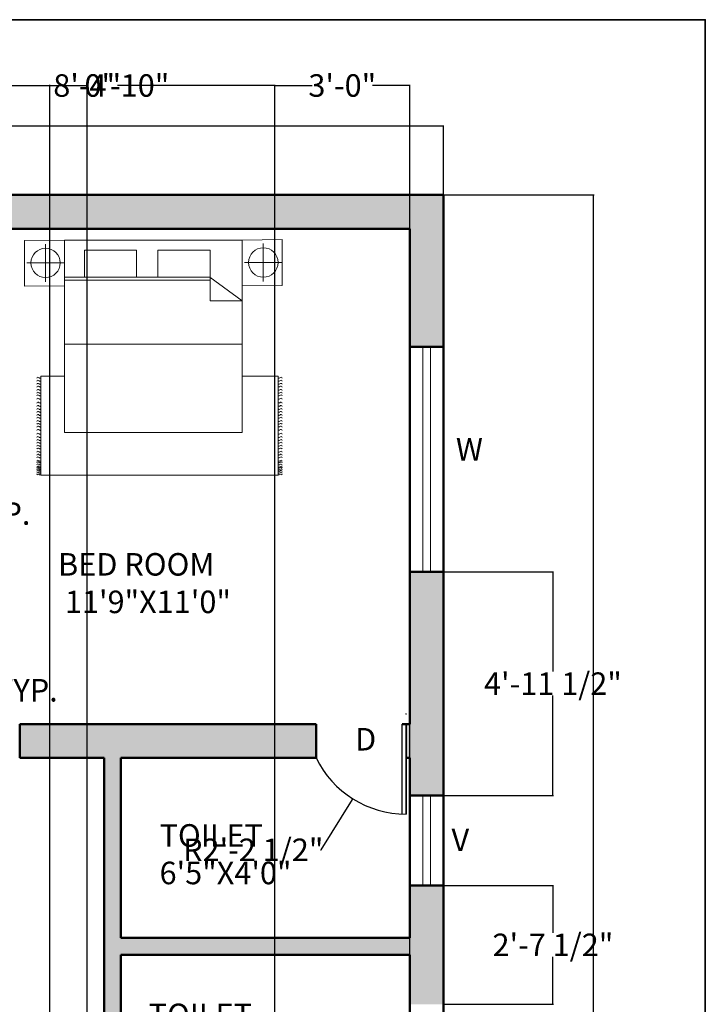
# Model space of a CAD drawing. Units: inches. Extents: x 125920 to 126336, y 366134 to 366735.
# Tile 6 of 6: x 126153 to 126336, y 366473 to 366735. Entities that reach past the tile are written whole.
import ezdxf

# ---------------------------------------------------------------- set-up
doc = ezdxf.new("R2010")
doc.units = ezdxf.units.IN
doc.header["$MEASUREMENT"] = 0
for name, color, linetype, lineweight in [('A-ANNO-DIMS', 2, 'Continuous', 18), ('A-ANNO-TEXT', 7, 'Continuous', 18), ('A-ANNO-TTLB', 7, 'Continuous', 35), ('A-AREA-IDEN', 7, 'Continuous', 25), ('A-DOOR', 3, 'Continuous', 25), ('A-FURN', 8, 'Continuous', 18), ('A-GLAZ', 4, 'Continuous', 18), ('A-WALL', 7, 'Continuous', 50)]:
    doc.layers.add(name, color=color, linetype=linetype, lineweight=lineweight)
doc.layers.add('A-WALL-PATT', color=18, linetype='Continuous', lineweight=13, true_color=0x000000)
doc.styles.get("Standard").update_dxf_attribs({"font": 'arial.ttf'})
doc.dimstyles.get("Standard").update_dxf_attribs({"dimtxt": 6, "dimasz": 0.18, "dimexe": 0.18, "dimexo": 0.0625, "dimgap": 0.09, "dimtad": 0, "dimtih": 1, "dimtoh": 1, "dimdec": 1, "dimzin": 0, "dimdsep": 46, "dimlunit": 3, "dimtxsty": 'Standard', "dimcen": 0.09, "dimadec": 0, "dimazin": 0, "dimtfac": 1, "dimtdec": 1, "dimtofl": 0, "dimtmove": 0, "dimatfit": 3, "dimfxl": 1, "dimtolj": 1, "dimtzin": 0, "dimarcsym": 0})

# ---------------------------------------------------------------- blocks, each defined once
blk = doc.blocks.new('*D3')
at = {"layer": 'A-ANNO-DIMS', "color": 0, "lineweight": -2, "transparency": 16777216}
for p, q in [((125966.47, 366688.86), (125966.47, 366707.25)), ((125966.65, 366707.07), (126111.24, 366707.07)), ((126266.29, 366707.07), (126121.71, 366707.07)), ((126266.47, 366688.86), (126266.47, 366707.25))]:
    blk.add_line(p, q, dxfattribs=at)
at = {"layer": 'A-ANNO-DIMS', "color": 0, "transparency": 16777216}
for points in [[(125966.65, 366707.1), (125966.65, 366707.04), (125966.47, 366707.07)], [(126266.29, 366707.1), (126266.29, 366707.04), (126266.47, 366707.07)]]:
    blk.add_solid(points, dxfattribs=at)
at = {"layer": 'Defpoints', "color": 0, "transparency": 16777216}
for p in [(126266.47, 366707.07), (125966.47, 366688.79), (126266.47, 366688.79)]:
    blk.add_point(p, dxfattribs=at)
at = {"layer": 'A-ANNO-DIMS', "color": 0, "transparency": 16777216, "insert": (126116.47, 366707.07), "char_height": 6, "attachment_point": 5}
blk.add_mtext("\\A1;25'", dxfattribs=at)
blk = doc.blocks.new('*D4')
at = {"layer": 'A-ANNO-DIMS', "color": 0, "lineweight": -2, "transparency": 16777216}
for p, q in [((126266.54, 366688.79), (126306.57, 366688.79)), ((126306.39, 366688.61), (126306.39, 366451.45)), ((126306.39, 366207.97), (126306.39, 366445.14)), ((126266.54, 366207.79), (126306.57, 366207.79))]:
    blk.add_line(p, q, dxfattribs=at)
at = {"layer": 'A-ANNO-DIMS', "color": 0, "transparency": 16777216}
for points in [[(126306.36, 366688.61), (126306.42, 366688.61), (126306.39, 366688.79)], [(126306.36, 366207.97), (126306.42, 366207.97), (126306.39, 366207.79)]]:
    blk.add_solid(points, dxfattribs=at)
at = {"layer": 'Defpoints', "color": 0, "transparency": 16777216}
for p in [(126266.47, 366688.79), (126266.47, 366207.79), (126306.39, 366207.79)]:
    blk.add_point(p, dxfattribs=at)
at = {"layer": 'A-ANNO-DIMS', "color": 0, "transparency": 16777216, "insert": (126306.39, 366448.29), "char_height": 6, "attachment_point": 5}
blk.add_mtext('\\A1;40\'-1.0"', dxfattribs=at)
blk = doc.blocks.new('BED-DOUBLE-WITH-NIGHTSTANDS')
for p, q in [((5.6, 61.62), (5.6, 51.56)), ((63.65, 61.72), (63.65, 51.66)), ((10.63, 56.59), (0.57, 56.59)), ((68.68, 56.69), (58.62, 56.69)), ((49.39, 52.82), (10.63, 52.82)), ((49.39, 52.82), (58, 46.47)), ((49.44, 52.82), (49.44, 46.47)), ((49.44, 52), (10.63, 52)), ((49.44, 46.47), (58, 46.47)), ((58.05, 34.96), (10.63, 34.96)), ((4.36, 0), (4.36, 26.37)), ((4.36, 26.37), (10.65, 26.37)), ((58.05, 26.37), (67.59, 26.37)), ((67.59, 26.37), (67.59, 0)), ((67.59, 0), (4.36, 0))]:
    blk.add_line(p, q)
for points in [[(0, 50.39), (10.63, 50.5), (10.63, 62.68), (0, 62.58)], [(58.05, 62.68), (58.05, 11.37), (10.63, 11.37), (10.63, 62.68)], [(58.05, 50.5), (68.68, 50.6), (68.68, 62.78), (58.05, 62.68)], [(29.88, 59.98), (29.88, 52.82), (15.98, 52.82), (15.98, 59.98)], [(49.44, 59.98), (49.44, 52.82), (35.55, 52.82), (35.55, 59.98)]]:
    blk.add_lwpolyline(points, close=True)
for centre in [(5.6, 56.59), (63.65, 56.69)]:
    blk.add_circle(centre, 3.92)
for points, knots in [([(3.23, 25.84), (3.32, 25.96), (3.52, 26.2), (3.86, 25.96), (4.14, 25.78), (4.29, 25.89), (4.36, 25.94)], [0, 0, 0, 0, 0.400747, 0.791423, 1.067667, 1.29709, 1.29709, 1.29709, 1.29709]), ([(3.23, 25.06), (3.32, 25.18), (3.52, 25.42), (3.86, 25.18), (4.14, 25.01), (4.29, 25.11), (4.36, 25.16)], [0, 0, 0, 0, 0.400747, 0.791423, 1.067667, 1.29709, 1.29709, 1.29709, 1.29709]), ([(3.23, 24.24), (3.32, 24.36), (3.52, 24.6), (3.86, 24.36), (4.14, 24.19), (4.29, 24.3), (4.36, 24.34)], [0, 0, 0, 0, 0.400747, 0.791423, 1.067667, 1.29709, 1.29709, 1.29709, 1.29709]), ([(3.23, 23.51), (3.32, 23.63), (3.52, 23.87), (3.86, 23.63), (4.14, 23.46), (4.29, 23.57), (4.36, 23.62)], [0, 0, 0, 0, 0.400747, 0.791423, 1.067667, 1.29709, 1.29709, 1.29709, 1.29709]), ([(68.71, 25.84), (68.61, 25.96), (68.42, 26.2), (68.08, 25.96), (67.8, 25.78), (67.65, 25.89), (67.58, 25.94)], [0, 0, 0, 0, 0.400747, 0.791423, 1.067667, 1.29709, 1.29709, 1.29709, 1.29709]), ([(68.71, 25.06), (68.61, 25.18), (68.42, 25.42), (68.08, 25.18), (67.8, 25.01), (67.65, 25.11), (67.58, 25.16)], [0, 0, 0, 0, 0.400747, 0.791423, 1.067667, 1.29709, 1.29709, 1.29709, 1.29709]), ([(68.71, 24.24), (68.61, 24.36), (68.42, 24.6), (68.08, 24.36), (67.8, 24.19), (67.65, 24.3), (67.58, 24.34)], [0, 0, 0, 0, 0.400747, 0.791423, 1.067667, 1.29709, 1.29709, 1.29709, 1.29709]), ([(68.71, 23.51), (68.61, 23.63), (68.42, 23.87), (68.08, 23.63), (67.8, 23.46), (67.65, 23.57), (67.58, 23.62)], [0, 0, 0, 0, 0.400747, 0.791423, 1.067667, 1.29709, 1.29709, 1.29709, 1.29709]), ([(3.23, 22.63), (3.32, 22.75), (3.52, 22.99), (3.86, 22.75), (4.14, 22.58), (4.29, 22.69), (4.36, 22.73)], [0, 0, 0, 0, 0.400747, 0.791423, 1.067667, 1.29709, 1.29709, 1.29709, 1.29709]), ([(3.23, 21.88), (3.32, 22), (3.52, 22.24), (3.86, 22), (4.14, 21.83), (4.29, 21.93), (4.36, 21.98)], [0, 0, 0, 0, 0.400747, 0.791423, 1.067667, 1.29709, 1.29709, 1.29709, 1.29709]), ([(3.23, 21.15), (3.32, 21.27), (3.52, 21.51), (3.86, 21.27), (4.14, 21.1), (4.29, 21.21), (4.36, 21.25)], [0, 0, 0, 0, 0.400747, 0.791423, 1.067667, 1.29709, 1.29709, 1.29709, 1.29709]), ([(68.71, 22.63), (68.61, 22.75), (68.42, 22.99), (68.08, 22.75), (67.8, 22.58), (67.65, 22.69), (67.58, 22.73)], [0, 0, 0, 0, 0.400747, 0.791423, 1.067667, 1.29709, 1.29709, 1.29709, 1.29709]), ([(68.71, 21.88), (68.61, 22), (68.42, 22.24), (68.08, 22), (67.8, 21.83), (67.65, 21.93), (67.58, 21.98)], [0, 0, 0, 0, 0.400747, 0.791423, 1.067667, 1.29709, 1.29709, 1.29709, 1.29709]), ([(68.71, 21.15), (68.61, 21.27), (68.42, 21.51), (68.08, 21.27), (67.8, 21.1), (67.65, 21.21), (67.58, 21.25)], [0, 0, 0, 0, 0.400747, 0.791423, 1.067667, 1.29709, 1.29709, 1.29709, 1.29709]), ([(3.23, 20.27), (3.32, 20.39), (3.52, 20.63), (3.86, 20.39), (4.14, 20.22), (4.29, 20.32), (4.36, 20.37)], [0, 0, 0, 0, 0.400747, 0.791423, 1.067667, 1.29709, 1.29709, 1.29709, 1.29709]), ([(3.23, 19.23), (3.32, 19.35), (3.52, 19.59), (3.86, 19.35), (4.14, 19.18), (4.29, 19.29), (4.36, 19.33)], [0, 0, 0, 0, 0.400747, 0.791423, 1.067667, 1.29709, 1.29709, 1.29709, 1.29709]), ([(3.23, 18.35), (3.32, 18.47), (3.52, 18.71), (3.86, 18.47), (4.14, 18.3), (4.29, 18.4), (4.36, 18.45)], [0, 0, 0, 0, 0.400747, 0.791423, 1.067667, 1.29709, 1.29709, 1.29709, 1.29709]), ([(68.71, 20.27), (68.61, 20.39), (68.42, 20.63), (68.08, 20.39), (67.8, 20.22), (67.65, 20.32), (67.58, 20.37)], [0, 0, 0, 0, 0.400747, 0.791423, 1.067667, 1.29709, 1.29709, 1.29709, 1.29709]), ([(68.71, 19.23), (68.61, 19.35), (68.42, 19.59), (68.08, 19.35), (67.8, 19.18), (67.65, 19.29), (67.58, 19.33)], [0, 0, 0, 0, 0.400747, 0.791423, 1.067667, 1.29709, 1.29709, 1.29709, 1.29709]), ([(68.71, 18.35), (68.61, 18.47), (68.42, 18.71), (68.08, 18.47), (67.8, 18.3), (67.65, 18.4), (67.58, 18.45)], [0, 0, 0, 0, 0.400747, 0.791423, 1.067667, 1.29709, 1.29709, 1.29709, 1.29709]), ([(3.23, 17.53), (3.32, 17.65), (3.52, 17.89), (3.86, 17.65), (4.14, 17.48), (4.29, 17.59), (4.36, 17.64)], [0, 0, 0, 0, 0.400747, 0.791423, 1.067667, 1.29709, 1.29709, 1.29709, 1.29709]), ([(3.23, 16.76), (3.32, 16.88), (3.52, 17.12), (3.86, 16.88), (4.14, 16.7), (4.29, 16.81), (4.36, 16.86)], [0, 0, 0, 0, 0.400747, 0.791423, 1.067667, 1.29709, 1.29709, 1.29709, 1.29709]), ([(3.23, 15.94), (3.32, 16.06), (3.52, 16.3), (3.86, 16.06), (4.14, 15.89), (4.29, 16), (4.36, 16.04)], [0, 0, 0, 0, 0.400747, 0.791423, 1.067667, 1.29709, 1.29709, 1.29709, 1.29709]), ([(68.71, 17.53), (68.61, 17.65), (68.42, 17.89), (68.08, 17.65), (67.8, 17.48), (67.65, 17.59), (67.58, 17.64)], [0, 0, 0, 0, 0.400747, 0.791423, 1.067667, 1.29709, 1.29709, 1.29709, 1.29709]), ([(68.71, 16.76), (68.61, 16.88), (68.42, 17.12), (68.08, 16.88), (67.8, 16.7), (67.65, 16.81), (67.58, 16.86)], [0, 0, 0, 0, 0.400747, 0.791423, 1.067667, 1.29709, 1.29709, 1.29709, 1.29709]), ([(68.71, 15.94), (68.61, 16.06), (68.42, 16.3), (68.08, 16.06), (67.8, 15.89), (67.65, 16), (67.58, 16.04)], [0, 0, 0, 0, 0.400747, 0.791423, 1.067667, 1.29709, 1.29709, 1.29709, 1.29709]), ([(3.23, 15.21), (3.32, 15.33), (3.52, 15.57), (3.86, 15.33), (4.14, 15.16), (4.29, 15.27), (4.36, 15.32)], [0, 0, 0, 0, 0.400747, 0.791423, 1.067667, 1.29709, 1.29709, 1.29709, 1.29709]), ([(3.23, 14.33), (3.32, 14.45), (3.52, 14.69), (3.86, 14.45), (4.14, 14.28), (4.29, 14.38), (4.36, 14.43)], [0, 0, 0, 0, 0.400747, 0.791423, 1.067667, 1.29709, 1.29709, 1.29709, 1.29709]), ([(3.23, 13.58), (3.32, 13.7), (3.52, 13.94), (3.86, 13.7), (4.14, 13.53), (4.29, 13.63), (4.36, 13.68)], [0, 0, 0, 0, 0.400747, 0.791423, 1.067667, 1.29709, 1.29709, 1.29709, 1.29709]), ([(3.23, 12.85), (3.32, 12.97), (3.52, 13.21), (3.86, 12.97), (4.14, 12.8), (4.29, 12.9), (4.36, 12.95)], [0, 0, 0, 0, 0.400747, 0.791423, 1.067667, 1.29709, 1.29709, 1.29709, 1.29709]), ([(68.71, 15.21), (68.61, 15.33), (68.42, 15.57), (68.08, 15.33), (67.8, 15.16), (67.65, 15.27), (67.58, 15.32)], [0, 0, 0, 0, 0.400747, 0.791423, 1.067667, 1.29709, 1.29709, 1.29709, 1.29709]), ([(68.71, 14.33), (68.61, 14.45), (68.42, 14.69), (68.08, 14.45), (67.8, 14.28), (67.65, 14.38), (67.58, 14.43)], [0, 0, 0, 0, 0.400747, 0.791423, 1.067667, 1.29709, 1.29709, 1.29709, 1.29709]), ([(68.71, 13.58), (68.61, 13.7), (68.42, 13.94), (68.08, 13.7), (67.8, 13.53), (67.65, 13.63), (67.58, 13.68)], [0, 0, 0, 0, 0.400747, 0.791423, 1.067667, 1.29709, 1.29709, 1.29709, 1.29709]), ([(68.71, 12.85), (68.61, 12.97), (68.42, 13.21), (68.08, 12.97), (67.8, 12.8), (67.65, 12.9), (67.58, 12.95)], [0, 0, 0, 0, 0.400747, 0.791423, 1.067667, 1.29709, 1.29709, 1.29709, 1.29709]), ([(3.23, 11.97), (3.32, 12.09), (3.52, 12.33), (3.86, 12.09), (4.14, 11.92), (4.29, 12.02), (4.36, 12.07)], [0, 0, 0, 0, 0.400747, 0.791423, 1.067667, 1.29709, 1.29709, 1.29709, 1.29709]), ([(3.23, 10.93), (3.32, 11.05), (3.52, 11.29), (3.86, 11.05), (4.14, 10.88), (4.29, 10.99), (4.36, 11.03)], [0, 0, 0, 0, 0.400747, 0.791423, 1.067667, 1.29709, 1.29709, 1.29709, 1.29709]), ([(68.71, 11.97), (68.61, 12.09), (68.42, 12.33), (68.08, 12.09), (67.8, 11.92), (67.65, 12.02), (67.58, 12.07)], [0, 0, 0, 0, 0.400747, 0.791423, 1.067667, 1.29709, 1.29709, 1.29709, 1.29709]), ([(68.71, 10.93), (68.61, 11.05), (68.42, 11.29), (68.08, 11.05), (67.8, 10.88), (67.65, 10.99), (67.58, 11.03)], [0, 0, 0, 0, 0.400747, 0.791423, 1.067667, 1.29709, 1.29709, 1.29709, 1.29709]), ([(3.23, 10.05), (3.32, 10.17), (3.52, 10.41), (3.86, 10.17), (4.14, 10), (4.29, 10.1), (4.36, 10.15)], [0, 0, 0, 0, 0.400747, 0.791423, 1.067667, 1.29709, 1.29709, 1.29709, 1.29709]), ([(3.23, 9.23), (3.32, 9.35), (3.52, 9.59), (3.86, 9.35), (4.14, 9.18), (4.29, 9.29), (4.36, 9.34)], [0, 0, 0, 0, 0.400747, 0.791423, 1.067667, 1.29709, 1.29709, 1.29709, 1.29709]), ([(3.23, 8.54), (3.32, 8.66), (3.52, 8.9), (3.86, 8.66), (4.14, 8.49), (4.29, 8.6), (4.36, 8.65)], [0, 0, 0, 0, 0.400747, 0.791423, 1.067667, 1.29709, 1.29709, 1.29709, 1.29709]), ([(3.23, 7.73), (3.32, 7.85), (3.52, 8.09), (3.86, 7.85), (4.14, 7.68), (4.29, 7.78), (4.36, 7.83)], [0, 0, 0, 0, 0.400747, 0.791423, 1.067667, 1.29709, 1.29709, 1.29709, 1.29709]), ([(68.71, 10.05), (68.61, 10.17), (68.42, 10.41), (68.08, 10.17), (67.8, 10), (67.65, 10.1), (67.58, 10.15)], [0, 0, 0, 0, 0.400747, 0.791423, 1.067667, 1.29709, 1.29709, 1.29709, 1.29709]), ([(68.71, 9.23), (68.61, 9.35), (68.42, 9.59), (68.08, 9.35), (67.8, 9.18), (67.65, 9.29), (67.58, 9.34)], [0, 0, 0, 0, 0.400747, 0.791423, 1.067667, 1.29709, 1.29709, 1.29709, 1.29709]), ([(68.71, 8.54), (68.61, 8.66), (68.42, 8.9), (68.08, 8.66), (67.8, 8.49), (67.65, 8.6), (67.58, 8.65)], [0, 0, 0, 0, 0.400747, 0.791423, 1.067667, 1.29709, 1.29709, 1.29709, 1.29709]), ([(68.71, 7.73), (68.61, 7.85), (68.42, 8.09), (68.08, 7.85), (67.8, 7.68), (67.65, 7.78), (67.58, 7.83)], [0, 0, 0, 0, 0.400747, 0.791423, 1.067667, 1.29709, 1.29709, 1.29709, 1.29709]), ([(3.23, 7), (3.32, 7.12), (3.52, 7.36), (3.86, 7.12), (4.14, 6.95), (4.29, 7.05), (4.36, 7.1)], [0, 0, 0, 0, 0.400747, 0.791423, 1.067667, 1.29709, 1.29709, 1.29709, 1.29709]), ([(3.23, 6.12), (3.32, 6.24), (3.52, 6.48), (3.86, 6.24), (4.14, 6.07), (4.29, 6.17), (4.36, 6.22)], [0, 0, 0, 0, 0.400747, 0.791423, 1.067667, 1.29709, 1.29709, 1.29709, 1.29709]), ([(3.23, 5.36), (3.32, 5.49), (3.52, 5.73), (3.86, 5.49), (4.14, 5.31), (4.29, 5.42), (4.36, 5.47)], [0, 0, 0, 0, 0.400747, 0.791423, 1.067667, 1.29709, 1.29709, 1.29709, 1.29709]), ([(68.71, 7), (68.61, 7.12), (68.42, 7.36), (68.08, 7.12), (67.8, 6.95), (67.65, 7.05), (67.58, 7.1)], [0, 0, 0, 0, 0.400747, 0.791423, 1.067667, 1.29709, 1.29709, 1.29709, 1.29709]), ([(68.71, 6.12), (68.61, 6.24), (68.42, 6.48), (68.08, 6.24), (67.8, 6.07), (67.65, 6.17), (67.58, 6.22)], [0, 0, 0, 0, 0.400747, 0.791423, 1.067667, 1.29709, 1.29709, 1.29709, 1.29709]), ([(68.71, 5.36), (68.61, 5.49), (68.42, 5.73), (68.08, 5.49), (67.8, 5.31), (67.65, 5.42), (67.58, 5.47)], [0, 0, 0, 0, 0.400747, 0.791423, 1.067667, 1.29709, 1.29709, 1.29709, 1.29709]), ([(3.23, 4.64), (3.32, 4.76), (3.52, 5), (3.86, 4.76), (4.14, 4.59), (4.29, 4.69), (4.36, 4.74)], [0, 0, 0, 0, 0.400747, 0.791423, 1.067667, 1.29709, 1.29709, 1.29709, 1.29709]), ([(3.23, 3.75), (3.32, 3.88), (3.52, 4.12), (3.86, 3.88), (4.14, 3.7), (4.29, 3.81), (4.36, 3.86)], [0, 0, 0, 0, 0.400747, 0.791423, 1.067667, 1.29709, 1.29709, 1.29709, 1.29709]), ([(3.23, 3.33), (3.32, 3.45), (3.52, 3.7), (3.86, 3.44), (4.14, 3.27), (4.29, 3.38), (4.36, 3.43)], [0, 0, 0, 0, 0.407265, 0.802015, 1.07826, 1.307683, 1.307683, 1.307683, 1.307683]), ([(3.23, 2.76), (3.32, 2.88), (3.52, 3.12), (3.86, 2.88), (4.14, 2.71), (4.29, 2.81), (4.36, 2.86)], [0, 0, 0, 0, 0.400747, 0.791423, 1.067667, 1.29709, 1.29709, 1.29709, 1.29709]), ([(68.71, 4.64), (68.61, 4.76), (68.42, 5), (68.08, 4.76), (67.8, 4.59), (67.66, 4.69), (67.59, 4.73)], [0, 0, 0, 0, 0.400747, 0.791423, 1.067667, 1.283686, 1.283686, 1.283686, 1.283686]), ([(68.71, 3.75), (68.61, 3.88), (68.42, 4.11), (68.08, 3.88), (67.8, 3.7), (67.66, 3.81), (67.59, 3.85)], [0, 0, 0, 0, 0.400747, 0.791423, 1.067667, 1.283686, 1.283686, 1.283686, 1.283686]), ([(68.71, 3.33), (68.61, 3.45), (68.42, 3.69), (68.08, 3.45), (67.8, 3.27), (67.66, 3.38), (67.59, 3.42)], [0, 0, 0, 0, 0.402903, 0.794912, 1.071156, 1.287177, 1.287177, 1.287177, 1.287177]), ([(68.71, 2.73), (68.61, 2.85), (68.42, 3.09), (68.08, 2.85), (67.8, 2.68), (67.66, 2.78), (67.59, 2.82)], [0, 0, 0, 0, 0.400747, 0.791423, 1.067667, 1.283686, 1.283686, 1.283686, 1.283686]), ([(3.23, 2.18), (3.32, 2.31), (3.52, 2.55), (3.86, 2.31), (4.14, 2.13), (4.29, 2.24), (4.36, 2.29)], [0, 0, 0, 0, 0.400747, 0.791423, 1.067667, 1.29709, 1.29709, 1.29709, 1.29709]), ([(3.23, 1.88), (3.32, 2), (3.52, 2.24), (3.86, 2), (4.14, 1.82), (4.29, 1.93), (4.36, 1.98)], [0, 0, 0, 0, 0.400747, 0.791423, 1.067667, 1.29709, 1.29709, 1.29709, 1.29709]), ([(3.23, 1.46), (3.32, 1.58), (3.52, 1.82), (3.86, 1.58), (4.14, 1.41), (4.29, 1.51), (4.36, 1.56)], [0, 0, 0, 0, 0.400747, 0.791423, 1.067667, 1.29709, 1.29709, 1.29709, 1.29709]), ([(3.23, 1.06), (3.32, 1.18), (3.52, 1.42), (3.86, 1.18), (4.14, 1.01), (4.29, 1.11), (4.36, 1.16)], [0, 0, 0, 0, 0.400747, 0.791423, 1.067667, 1.29709, 1.29709, 1.29709, 1.29709]), ([(3.23, 0.57), (3.32, 0.7), (3.52, 0.94), (3.86, 0.7), (4.14, 0.52), (4.29, 0.63), (4.36, 0.68)], [0, 0, 0, 0, 0.400747, 0.791423, 1.067667, 1.29709, 1.29709, 1.29709, 1.29709]), ([(3.23, 0.07), (3.32, 0.19), (3.52, 0.43), (3.86, 0.19), (4.14, 0.02), (4.29, 0.13), (4.36, 0.18)], [0, 0, 0, 0, 0.400747, 0.791423, 1.067667, 1.29709, 1.29709, 1.29709, 1.29709]), ([(68.71, 1.43), (68.61, 1.55), (68.42, 1.79), (68.08, 1.55), (67.8, 1.38), (67.65, 1.48), (67.58, 1.53)], [0, 0, 0, 0, 0.400747, 0.791423, 1.067667, 1.29709, 1.29709, 1.29709, 1.29709]), ([(68.71, 1.03), (68.61, 1.15), (68.42, 1.39), (68.08, 1.15), (67.8, 0.98), (67.65, 1.09), (67.58, 1.13)], [0, 0, 0, 0, 0.400747, 0.791423, 1.067667, 1.29709, 1.29709, 1.29709, 1.29709]), ([(68.71, 0.55), (68.61, 0.67), (68.42, 0.91), (68.08, 0.67), (67.8, 0.49), (67.65, 0.6), (67.58, 0.65)], [0, 0, 0, 0, 0.400747, 0.791423, 1.067667, 1.29709, 1.29709, 1.29709, 1.29709]), ([(68.71, 0.07), (68.61, 0.19), (68.42, 0.43), (68.08, 0.19), (67.8, 0.02), (67.65, 0.13), (67.58, 0.18)], [0, 0, 0, 0, 0.400747, 0.791423, 1.067667, 1.29709, 1.29709, 1.29709, 1.29709]), ([(68.71, 2.16), (68.61, 2.28), (68.42, 2.52), (68.08, 2.28), (67.8, 2.11), (67.66, 2.21), (67.59, 2.25)], [0, 0, 0, 0, 0.400747, 0.791423, 1.067667, 1.283686, 1.283686, 1.283686, 1.283686]), ([(68.71, 1.85), (68.61, 1.97), (68.42, 2.21), (68.08, 1.97), (67.8, 1.8), (67.66, 1.9), (67.59, 1.94)], [0, 0, 0, 0, 0.400747, 0.791423, 1.067667, 1.283686, 1.283686, 1.283686, 1.283686])]:
    blk.add_open_spline(points, degree=3, knots=knots)
blk = doc.blocks.new('WIN-60')
for p, q in [((0, 0), (0, 60)), ((3.5, 0), (3.5, 60)), ((5.5, 60), (5.5, 0)), ((9, 60), (9, 0))]:
    blk.add_line(p, q)
blk = doc.blocks.new('VENT-24')
for p, q in [((0, 0), (0, 24)), ((3.5, 0), (3.5, 24)), ((5.5, 24), (5.5, 0)), ((9, 24), (9, 0))]:
    blk.add_line(p, q)
blk = doc.blocks.new('*D19')
at = {"layer": 'A-ANNO-DIMS', "color": 0, "lineweight": -2, "transparency": 16777216}
for p, q in [((126000.69, 366614.13), (126000.69, 366603.71)), ((126069.4, 366614.13), (126069.4, 366603.71)), ((126000.87, 366603.89), (126069.22, 366603.89)), ((126069.4, 366603.89), (126069.58, 366603.89))]:
    blk.add_line(p, q, dxfattribs=at)
at = {"layer": 'A-ANNO-DIMS', "color": 0, "transparency": 16777216}
for points in [[(126000.87, 366603.92), (126000.87, 366603.86), (126000.69, 366603.89)], [(126069.22, 366603.92), (126069.22, 366603.86), (126069.4, 366603.89)]]:
    blk.add_solid(points, dxfattribs=at)
at = {"layer": 'Defpoints', "color": 0, "transparency": 16777216}
for p in [(126000.69, 366614.19), (126069.4, 366614.19), (126069.4, 366603.89)]:
    blk.add_point(p, dxfattribs=at)
at = {"layer": 'A-ANNO-DIMS', "color": 0, "transparency": 16777216, "insert": (126113.91, 366603.89), "char_height": 6, "attachment_point": 5}
blk.add_mtext('\\A1;BED SET 5\'-8 1/2" TYP.', dxfattribs=at)
blk = doc.blocks.new('*D25')
at = {"layer": 'A-ANNO-DIMS', "color": 0, "lineweight": -2, "transparency": 16777216}
for p, q in [((126117.41, 366574.79), (126111.89, 366574.79)), ((126112.07, 366574.61), (126112.07, 366559.99)), ((126112.07, 366538.97), (126112.07, 366553.6)), ((126117.41, 366538.79), (126111.89, 366538.79))]:
    blk.add_line(p, q, dxfattribs=at)
at = {"layer": 'A-ANNO-DIMS', "color": 0, "transparency": 16777216}
for points in [[(126112.04, 366574.61), (126112.1, 366574.61), (126112.07, 366574.79)], [(126112.04, 366538.97), (126112.1, 366538.97), (126112.07, 366538.79)]]:
    blk.add_solid(points, dxfattribs=at)
at = {"layer": 'Defpoints', "color": 0, "transparency": 16777216}
for p in [(126112.07, 366574.79), (126117.47, 366574.79), (126117.47, 366538.79)]:
    blk.add_point(p, dxfattribs=at)
at = {"layer": 'A-ANNO-DIMS', "color": 0, "transparency": 16777216, "insert": (126112.07, 366556.79), "char_height": 6, "attachment_point": 5}
blk.add_mtext('\\A1;BEDROOM DOOR 3\'-0" TYP.', dxfattribs=at)
blk = doc.blocks.new('*D34')
at = {"layer": 'A-ANNO-DIMS', "color": 0, "lineweight": -2, "transparency": 16777216}
for p, q in [((126266.54, 366504.78), (126295.8, 366504.78)), ((126295.62, 366504.6), (126295.62, 366492.13)), ((126295.62, 366473.28), (126295.62, 366485.75)), ((126266.54, 366473.1), (126295.8, 366473.1))]:
    blk.add_line(p, q, dxfattribs=at)
at = {"layer": 'A-ANNO-DIMS', "color": 0, "transparency": 16777216}
for points in [[(126295.59, 366504.6), (126295.65, 366504.6), (126295.62, 366504.78)], [(126295.59, 366473.28), (126295.65, 366473.28), (126295.62, 366473.1)]]:
    blk.add_solid(points, dxfattribs=at)
at = {"layer": 'Defpoints', "color": 0, "transparency": 16777216}
for p in [(126266.47, 366504.78), (126295.62, 366504.78), (126266.47, 366473.1)]:
    blk.add_point(p, dxfattribs=at)
at = {"layer": 'A-ANNO-DIMS', "color": 0, "transparency": 16777216, "insert": (126295.62, 366488.94), "char_height": 6, "attachment_point": 5}
blk.add_mtext('\\A1;2\'-7 1/2"', dxfattribs=at)
blk = doc.blocks.new('*D35')
at = {"layer": 'A-ANNO-DIMS', "color": 0, "lineweight": -2, "transparency": 16777216}
for p, q in [((126266.54, 366588.33), (126295.8, 366588.33)), ((126295.62, 366588.15), (126295.62, 366561.75)), ((126295.62, 366528.96), (126295.62, 366555.36)), ((126266.54, 366528.78), (126295.8, 366528.78))]:
    blk.add_line(p, q, dxfattribs=at)
at = {"layer": 'A-ANNO-DIMS', "color": 0, "transparency": 16777216}
for points in [[(126295.59, 366588.15), (126295.65, 366588.15), (126295.62, 366588.33)], [(126295.59, 366528.96), (126295.65, 366528.96), (126295.62, 366528.78)]]:
    blk.add_solid(points, dxfattribs=at)
at = {"layer": 'Defpoints', "color": 0, "transparency": 16777216}
for p in [(126266.47, 366588.33), (126295.62, 366588.33), (126266.47, 366528.78)]:
    blk.add_point(p, dxfattribs=at)
at = {"layer": 'A-ANNO-DIMS', "color": 0, "transparency": 16777216, "insert": (126295.62, 366558.55), "char_height": 6, "attachment_point": 5}
blk.add_mtext('\\A1;4\'-11 1/2"', dxfattribs=at)
blk = doc.blocks.new('*D41')
at = {"layer": 'A-ANNO-DIMS', "color": 0, "lineweight": -2, "transparency": 16777216}
for p, q in [((126121.47, 366216.86), (126121.47, 366718.12)), ((126121.65, 366717.94), (126163.4, 366717.94)), ((126221.29, 366717.94), (126179.54, 366717.94)), ((126221.47, 366216.86), (126221.47, 366718.12))]:
    blk.add_line(p, q, dxfattribs=at)
at = {"layer": 'A-ANNO-DIMS', "color": 0, "transparency": 16777216}
for points in [[(126121.65, 366717.97), (126121.65, 366717.91), (126121.47, 366717.94)], [(126221.29, 366717.97), (126221.29, 366717.91), (126221.47, 366717.94)]]:
    blk.add_solid(points, dxfattribs=at)
at = {"layer": 'Defpoints', "color": 0, "transparency": 16777216}
for p in [(126221.47, 366717.94), (126121.47, 366216.79), (126221.47, 366216.79)]:
    blk.add_point(p, dxfattribs=at)
at = {"layer": 'A-ANNO-DIMS', "color": 0, "transparency": 16777216, "insert": (126171.47, 366717.94), "char_height": 6, "attachment_point": 5}
blk.add_mtext('\\A1;8\'-4"', dxfattribs=at)
blk = doc.blocks.new('*D43')
at = {"layer": 'A-ANNO-DIMS', "color": 0, "lineweight": -2, "transparency": 16777216}
for p, q in [((126221.47, 366216.86), (126221.47, 366718.12)), ((126221.65, 366717.94), (126231.41, 366717.94)), ((126257.29, 366717.94), (126247.54, 366717.94)), ((126257.47, 366216.86), (126257.47, 366718.12))]:
    blk.add_line(p, q, dxfattribs=at)
at = {"layer": 'A-ANNO-DIMS', "color": 0, "transparency": 16777216}
for points in [[(126221.65, 366717.97), (126221.65, 366717.91), (126221.47, 366717.94)], [(126257.29, 366717.97), (126257.29, 366717.91), (126257.47, 366717.94)]]:
    blk.add_solid(points, dxfattribs=at)
at = {"layer": 'Defpoints', "color": 0, "transparency": 16777216}
for p in [(126257.47, 366717.94), (126221.47, 366216.79), (126257.47, 366216.79)]:
    blk.add_point(p, dxfattribs=at)
at = {"layer": 'A-ANNO-DIMS', "color": 0, "transparency": 16777216, "insert": (126239.47, 366717.94), "char_height": 6, "attachment_point": 5}
blk.add_mtext('\\A1;3\'-0"', dxfattribs=at)
blk = doc.blocks.new('*D44')
at = {"layer": 'A-ANNO-DIMS', "color": 0, "lineweight": -2, "transparency": 16777216}
for p, q in [((126161.47, 366252.86), (126161.47, 366718.12)), ((126161.65, 366717.94), (126171.29, 366717.94)), ((126171.47, 366252.86), (126171.47, 366718.12)), ((126171.47, 366717.94), (126171.65, 366717.94))]:
    blk.add_line(p, q, dxfattribs=at)
at = {"layer": 'A-ANNO-DIMS', "color": 0, "transparency": 16777216}
for points in [[(126161.65, 366717.97), (126161.65, 366717.91), (126161.47, 366717.94)], [(126171.29, 366717.97), (126171.29, 366717.91), (126171.47, 366717.94)]]:
    blk.add_solid(points, dxfattribs=at)
at = {"layer": 'Defpoints', "color": 0, "transparency": 16777216}
for p in [(126171.47, 366717.94), (126161.47, 366252.79), (126171.47, 366252.79)]:
    blk.add_point(p, dxfattribs=at)
at = {"layer": 'A-ANNO-DIMS', "color": 0, "transparency": 16777216, "insert": (126182.05, 366717.94), "char_height": 6, "attachment_point": 5}
blk.add_mtext('\\A1;0\'-10"', dxfattribs=at)
blk = doc.blocks.new('*D50')
at = {"layer": 'A-ANNO-DIMS', "color": 0, "lineweight": -2, "transparency": 16777216}
for p, q in [((126256.38, 366550.49), (126256.56, 366550.49)), ((126256.47, 366550.4), (126256.47, 366550.58)), ((126233.83, 366514.27), (126242.23, 366527.7)), ((126233.65, 366514.27), (126233.83, 366514.27))]:
    blk.add_line(p, q, dxfattribs=at)
at = {"layer": 'A-ANNO-DIMS', "color": 0, "transparency": 16777216}
blk.add_solid([(126242.2, 366527.72), (126242.25, 366527.68), (126242.32, 366527.85)], dxfattribs=at)
at = {"layer": 'Defpoints', "color": 0, "transparency": 16777216}
for p in [(126256.47, 366550.49), (126242.32, 366527.85)]:
    blk.add_point(p, dxfattribs=at)
at = {"layer": 'A-ANNO-DIMS', "color": 0, "transparency": 16777216, "insert": (126215.73, 366514.27), "char_height": 6, "attachment_point": 5}
blk.add_mtext('\\A1;R2\'-2 1/2"', dxfattribs=at)

msp = doc.modelspace()

# ---------------------------------------------------------------- hatches: boundary and pattern name
at = {"layer": 'A-WALL-PATT'}
h = msp.add_hatch(color=256, dxfattribs=at)
h.dxf.hatch_style = 1
h.paths.add_polyline_path([(126266.47, 366688.79), (125966.47, 366688.79), (125966.47, 366649.55), (125975.47, 366649.55), (125975.47, 366679.79), (126107.47, 366679.79), (126107.47, 366547.79), (126106.47, 366547.79), (126106.47, 366538.79), (126107.47, 366538.79), (126117.47, 366538.79), (126117.47, 366547.79), (126116.47, 366547.79), (126116.47, 366679.79), (126257.47, 366679.79), (126257.47, 366648.33), (126266.47, 366648.33)])
h.paths.add_polyline_path([(126070.47, 366547.79), (125975.47, 366547.79), (125975.47, 366589.55), (125966.47, 366589.55), (125966.47, 366528.42), (125975.47, 366528.42), (125975.47, 366538.79), (126059.47, 366538.79), (126059.47, 366515.79), (126063.97, 366515.79), (126063.97, 366538.79), (126070.47, 366538.79)])
h.paths.add_polyline_path([(125975.47, 366486.29), (126063.97, 366486.29), (126063.97, 366491.79), (126059.47, 366491.79), (126059.47, 366490.79), (125975.47, 366490.79), (125975.47, 366504.42), (125966.47, 366504.42), (125966.47, 366437.07), (125975.47, 366437.07)])
h.paths.add_polyline_path([(125975.47, 366312.79), (126022.47, 366312.79), (126022.47, 366317.29), (125975.47, 366317.29), (125975.47, 366377.07), (125966.47, 366377.07), (125966.47, 366207.79), (125987.64, 366207.79), (125987.64, 366216.79), (125975.47, 366216.79)])
h.paths.add_polyline_path([(126063.97, 366216.79), (126063.97, 366312.79), (126070.47, 366312.79), (126070.47, 366317.29), (126058.47, 366317.29), (126058.47, 366312.79), (126059.47, 366312.79), (126059.47, 366216.79), (126047.64, 366216.79), (126047.64, 366207.79), (126063.97, 366207.79)])
h.paths.add_polyline_path([(126221.47, 366216.79), (126116.47, 366216.79), (126107.47, 366216.79), (126107.47, 366207.79), (126221.47, 366207.79)])
h.paths.add_polyline_path([(126266.47, 366336.48), (126257.47, 366336.48), (126257.47, 366297.79), (126174.23, 366297.79), (126174.23, 366288.79), (126257.47, 366288.79), (126257.47, 366207.79), (126266.47, 366207.79)])
h.paths.add_polyline_path([(126138.23, 366297.79), (126116.47, 366297.79), (126116.47, 366433.79), (126117.47, 366433.79), (126117.47, 366438.29), (126116.47, 366438.29), (126107.47, 366438.29), (126107.47, 366317.29), (126106.47, 366317.29), (126106.47, 366312.79), (126107.47, 366312.79), (126107.47, 366288.79), (126116.47, 366288.79), (126138.23, 366288.79)])
h.paths.add_polyline_path([(126266.47, 366449.1), (126257.47, 366449.1), (126257.47, 366438.29), (126256.47, 366438.29), (126256.47, 366433.79), (126257.47, 366433.79), (126257.47, 366396.48), (126266.47, 366396.48)])
h.paths.add_polyline_path([(126232.47, 366438.29), (126180.47, 366438.29), (126180.47, 366486.29), (126257.47, 366486.29), (126257.47, 366473.1), (126266.47, 366473.1), (126266.47, 366504.78), (126257.47, 366504.78), (126257.47, 366490.79), (126180.47, 366490.79), (126180.47, 366538.79), (126232.47, 366538.79), (126232.47, 366547.79), (126153.47, 366547.79), (126153.47, 366538.79), (126175.97, 366538.79), (126175.97, 366438.29), (126153.47, 366438.29), (126153.47, 366433.79), (126232.47, 366433.79)])
h.paths.add_polyline_path([(126266.47, 366588.33), (126257.47, 366588.33), (126257.47, 366547.79), (126256.47, 366547.79), (126256.47, 366538.79), (126257.47, 366538.79), (126257.47, 366528.78), (126266.47, 366528.78)])

# ---------------------------------------------------------------- linework, layer by layer
at = {"layer": 'A-ANNO-TTLB'}
msp.add_lwpolyline([(125932.73, 366735.48), (126336.24, 366735.48), (126336.24, 366133.52), (125932.73, 366133.52)], close=True, dxfattribs=at)
at = {"layer": 'A-DOOR'}
for p, q in [((126256.47, 366547.79), (126255.47, 366547.79)), ((126255.47, 366523.79), (126255.47, 366547.79)), ((126257.47, 366547.79), (126256.47, 366547.79)), ((126256.47, 366547.79), (126256.47, 366523.79)), ((126256.47, 366523.79), (126256.47, 366547.79))]:
    msp.add_line(p, q, dxfattribs=at)
msp.add_arc((126256.47, 366550.49), 26.7, 205.9892, 270, dxfattribs=at)
at = {"layer": 'A-WALL'}
for p, q in [((125966.47, 366688.79), (126266.47, 366688.79)), ((126266.47, 366688.79), (126266.47, 366207.79)), ((126116.47, 366679.79), (126257.47, 366679.79)), ((126257.47, 366679.79), (126257.47, 366547.79)), ((126257.47, 366648.33), (126266.47, 366648.33)), ((126266.47, 366588.33), (126257.47, 366588.33)), ((126153.47, 366538.79), (126153.47, 366547.79)), ((126153.47, 366547.79), (126232.47, 366547.79)), ((126232.47, 366547.79), (126232.47, 366538.79)), ((126255.47, 366547.79), (126257.47, 366547.79)), ((126153.47, 366538.79), (126175.97, 366538.79)), ((126175.97, 366538.79), (126175.97, 366438.29)), ((126180.47, 366538.79), (126180.47, 366490.79)), ((126180.47, 366538.79), (126232.47, 366538.79)), ((126256.47, 366538.79), (126257.47, 366538.79)), ((126257.47, 366538.79), (126257.47, 366490.79)), ((126257.47, 366528.78), (126266.47, 366528.78)), ((126266.47, 366504.78), (126257.47, 366504.78)), ((126180.47, 366490.79), (126257.47, 366490.79)), ((126180.47, 366490.79), (126257.47, 366490.79)), ((126180.47, 366486.29), (126257.47, 366486.29)), ((126180.47, 366486.29), (126257.47, 366486.29)), ((126180.47, 366486.29), (126180.47, 366438.29)), ((126257.47, 366486.29), (126257.47, 366438.29))]:
    msp.add_line(p, q, dxfattribs=at)

# ---------------------------------------------------------------- block references
at = {"layer": 'A-FURN'}
msp.add_blockref('BED-DOUBLE-WITH-NIGHTSTANDS', (126154.77, 366614.08), dxfattribs=at)
at = {"layer": 'A-GLAZ'}
for name, p in [('WIN-60', (126257.47, 366588.33)), ('VENT-24', (126257.47, 366504.78))]:
    msp.add_blockref(name, p, dxfattribs=at)

# ---------------------------------------------------------------- texts
at = {"layer": 'A-ANNO-TEXT', "char_height": 6, "attachment_point": 1}
for s, width, insert in [('W', 14.507, (126269.76, 366624)), ('D', 9.6923, (126242.88, 366546.73)), ('V', 9.8961, (126268.58, 366519.91))]:
    msp.add_mtext_dynamic_manual_height_columns(s, width=width, gutter_width=30, heights=[0], dxfattribs=dict(at, insert=insert))
at = {"layer": 'A-AREA-IDEN', "char_height": 6, "attachment_point": 1}
for s, width, insert in [('BED ROOM\\P 11\'9"X11\'0"', 56.7294, (126163.7, 366593.34)), ('TOILET\\P6\'5"X4\'0"', 50.3567, (126190.76, 366521.1)), ('TOILET\\P6\'5"X4\'0"', 40.1985, (126187.86, 366473.28))]:
    msp.add_mtext_dynamic_manual_height_columns(s, width=width, gutter_width=30, heights=[0], dxfattribs=dict(at, insert=insert))

# ---------------------------------------------------------------- dimensions: what is measured, and where the dimension line sits
at = {"layer": 'A-ANNO-DIMS'}
for base, p1, p2, override, picture, middle in [((126221.47, 366717.94), (126121.47, 366216.79), (126221.47, 366216.79), {"dimdec": 1, "dimlfac": 1, "dimrnd": 0, "dimzin": 1, "dimdsep": 46, "dimlunit": 4, "dimfrac": 2}, '*D41', (126171.47, 366717.94)), ((126171.47, 366717.94), (126161.47, 366252.79), (126171.47, 366252.79), {"dimdec": 1, "dimlfac": 1, "dimrnd": 0, "dimzin": 1, "dimdsep": 46, "dimlunit": 4, "dimfrac": 2}, '*D44', (126182.05, 366717.94)), ((126257.47, 366717.94), (126221.47, 366216.79), (126257.47, 366216.79), {"dimdec": 1, "dimlfac": 1, "dimrnd": 0, "dimzin": 1, "dimdsep": 46, "dimlunit": 4, "dimfrac": 2}, '*D43', (126239.47, 366717.94)), ((126266.47, 366707.07), (125966.47, 366688.79), (126266.47, 366688.79), {"dimclrd": 0, "dimclre": 0, "dimclrt": 0}, '*D3', (126116.47, 366707.07))]:
    dim = msp.add_linear_dim(base=base, p1=p1, p2=p2, dimstyle='Standard', override=override, dxfattribs=at)
    dim.commit()
    dim.dimension.update_dxf_attribs({"geometry": picture, "text_midpoint": middle})
for base, p1, p2, override, picture, middle in [((126306.39, 366207.79), (126266.47, 366688.79), (126266.47, 366207.79), {"dimclrd": 0, "dimclre": 0, "dimclrt": 0}, '*D4', (126306.39, 366448.29)), ((126295.6231, 366588.3315), (126266.4731, 366528.7777), (126266.4731, 366588.3315), {"dimdec": 1, "dimlfac": 1, "dimrnd": 0, "dimzin": 1, "dimdsep": 46, "dimlunit": 4, "dimfrac": 2}, '*D35', (126295.6231, 366558.5546)), ((126295.62, 366504.78), (126266.47, 366473.1), (126266.47, 366504.78), {"dimdec": 1, "dimlfac": 1, "dimrnd": 0, "dimzin": 1, "dimdsep": 46, "dimlunit": 4, "dimfrac": 2}, '*D34', (126295.62, 366488.94))]:
    dim = msp.add_linear_dim(base=base, p1=p1, p2=p2, angle=90, dimstyle='Standard', override=override, dxfattribs=at)
    dim.commit()
    dim.dimension.update_dxf_attribs({"geometry": picture, "text_midpoint": middle})
dim = msp.add_linear_dim(base=(126069.4, 366603.89), p1=(126000.69, 366614.19), p2=(126069.4, 366614.19), text='BED SET <> TYP.', dimstyle='Standard', override={"dimdec": 1, "dimlfac": 1, "dimrnd": 0, "dimzin": 1, "dimdsep": 46, "dimlunit": 4, "dimfrac": 2}, dxfattribs=at)
dim.commit()
dim.dimension.update_dxf_attribs({"geometry": '*D19', "text_midpoint": (126113.91, 366603.89)})
dim = msp.add_linear_dim(base=(126112.07, 366574.79), p1=(126117.47, 366538.79), p2=(126117.47, 366574.79), angle=90, text='BEDROOM DOOR <> TYP.', dimstyle='Standard', override={"dimdec": 1, "dimlfac": 1, "dimrnd": 0, "dimzin": 1, "dimdsep": 46, "dimlunit": 4, "dimfrac": 2}, dxfattribs=at)
dim.commit()
dim.dimension.update_dxf_attribs({"geometry": '*D25', "text_midpoint": (126112.07, 366556.79)})
dim = msp.add_radius_dim(center=(126256.47, 366550.49), mpoint=(126242.32, 366527.85), dimstyle='Standard', override={"dimdec": 1, "dimlfac": 1, "dimrnd": 0, "dimzin": 1, "dimdsep": 46, "dimlunit": 4, "dimfrac": 2}, dxfattribs=at)
dim.commit()
dim.dimension.update_dxf_attribs({"geometry": '*D50', "text_midpoint": (126215.73, 366514.27), "dimtype": 164})

doc.saveas('drawing.dxf')
